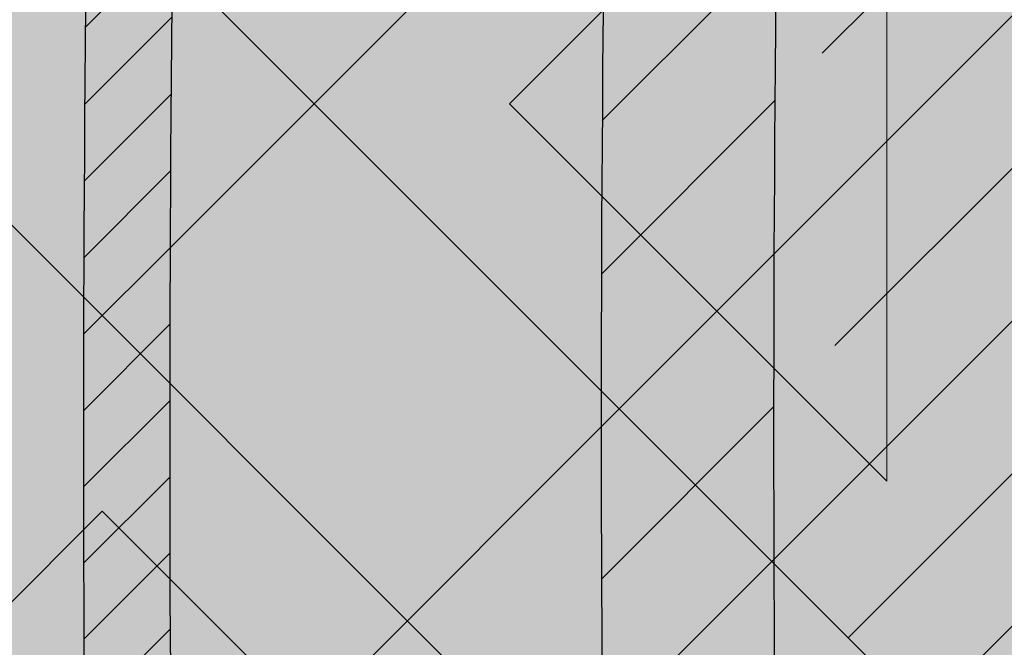
# Model space of a CAD drawing. Units: inches. Extents: x 844 to 2234, y 346 to 1084.
# Tile 11 of 93: x 1119.118 to 1120.937, y 693.702 to 694.861. Entities that reach past the tile are written whole.
import ezdxf

# ---------------------------------------------------------------- set-up
doc = ezdxf.new("R2010")
doc.units = ezdxf.units.IN
doc.header["$MEASUREMENT"] = 0
for name, color, linetype, lineweight in [('A-ANNO-DIMS', 2, 'Continuous', 18), ('furniture', 8, 'Continuous', 18), ('RA-AP-01$0$INT', 35, 'Continuous', 5)]:
    doc.layers.add(name, color=color, linetype=linetype, lineweight=lineweight)
doc.layers.add('RA-AP-01$0$FURN', color=3, linetype='Continuous')
doc.layers.add('RA-AP-01$0$WOOD', color=64, linetype='Continuous')
doc.styles.get("Standard").update_dxf_attribs({"font": 'arial.ttf'})
doc.dimstyles.get("Standard").update_dxf_attribs({"dimtxt": 6, "dimasz": 3, "dimexe": 0.18, "dimexo": 0.0625, "dimgap": 0.09, "dimtad": 0, "dimtih": 1, "dimtoh": 1, "dimdec": 1, "dimzin": 0, "dimdsep": 46, "dimlunit": 3, "dimtxsty": 'Standard', "dimblk": 'ARCHTICK', "dimcen": 0.09, "dimadec": 0, "dimazin": 0, "dimtfac": 1, "dimtdec": 1, "dimtofl": 0, "dimtmove": 0, "dimatfit": 3, "dimfxl": 1, "dimtolj": 1, "dimtzin": 0, "dimarcsym": 0})

# ---------------------------------------------------------------- blocks, each defined once
blk = doc.blocks.new('A$C18D01794')
at = {"layer": 'RA-AP-01$0$INT'}
h = blk.add_hatch(color=256, dxfattribs=at)
h.paths.add_polyline_path([(4.585917135068449, -6.356712009588271), (4.555206456959269, -6.35671200958746), (4.555206456959137, -6.387422687716308), (4.874495778835233, -6.706712009592356), (4.90520645695423, -6.676001331474049)])
h.paths.add_polyline_path([(5.255206456948813, -6.387422687716306), (5.255206456948682, -6.356712009605972), (5.224495778822613, -6.356712009605161), (4.905206456953498, -6.676001331474273), (4.935917135072151, -6.706712009592924)])
h.paths.add_polyline_path([(4.935917135072559, -6.706712009592068), (4.905206456953564, -6.737422687710376), (5.255206456951813, -7.087422687708613), (5.255206456951549, -7.026001331471008)])
h.paths.add_polyline_path([(4.555206456956399, -7.026001331471013), (4.555206456956134, -7.087422687708616), (4.905206456953821, -6.737422687710943), (4.874495778835166, -6.70671200959229)])
h = blk.add_hatch(color=256, dxfattribs=at)
h.paths.add_polyline_path([(4.585917135068448, -6.356712009588273), (4.614201406330596, -6.356712009589021), (4.668846067270487, -6.411356670531338), (4.723490728212344, -6.356712009591912), (4.771774999457151, -6.35671200959319), (4.826419660396886, -6.411356670535356), (4.862780050090322, -6.374996280843536), (4.844495778842715, -6.356712009595112), (4.862780050090411, -6.356712009595595), (4.905206456960182, -6.399138416468211), (4.947632863832445, -6.356712009597838), (4.965917135079675, -6.356712009598322), (4.947632863831759, -6.374996280845421), (4.983993253523576, -6.411356670538857), (5.038637914464627, -6.356712009600247), (5.08692218571208, -6.356712009601523), (5.141566846649976, -6.411356670541852), (5.196211507589851, -6.356712009604411), (5.224495778822615, -6.356712009605161), (4.905206456953975, -6.676001331473793)])
h.paths.add_polyline_path([(4.895206456956031, -6.637717060225675), (4.895206456958921, -6.528427738347902), (4.840561796018589, -6.583072399285802)], flags=16)
h.paths.add_polyline_path([(4.915206456955638, -6.637717060226121), (4.969851117895509, -6.583072399288678), (4.915206456957609, -6.528427738348344)], flags=16)
h.paths.add_polyline_path([(4.826419660395175, -6.568930263661755), (4.881064321335613, -6.514285602723745), (4.771774999456703, -6.514285602720857)], flags=16)
h.paths.add_polyline_path([(4.983993253519558, -6.568930263665262), (5.038637914460456, -6.514285602726792), (4.929348592581548, -6.514285602724816)], flags=16)
h.paths.add_polyline_path([(4.881064321336025, -6.494285602723742), (4.826419660397532, -6.439640941782821), (4.771774999457062, -6.494285602720859)], flags=16)
h.paths.add_polyline_path([(4.929348592582019, -6.494285602724817), (5.038637914460982, -6.494285602726792), (4.983993253522945, -6.439640941786327)], flags=16)
h.paths.add_polyline_path([(4.895206456960191, -6.480143467100443), (4.895206456962115, -6.407422687715913), (4.876922185715016, -6.389138416467584), (4.840561796021581, -6.425498806159401)], flags=16)
h.paths.add_polyline_path([(4.915206456958487, -6.480143467100889), (4.969851117899527, -6.425498806162279), (4.933490728206909, -6.389138416468043), (4.9152064569598, -6.40742268771434)], flags=16)
h.paths.add_polyline_path([(4.757632863832376, -6.480143467096812), (4.812277524772842, -6.425498806158772), (4.757632863834348, -6.370854145217844)], flags=16)
h.paths.add_polyline_path([(4.737632863832376, -6.480143467096286), (4.737632863834348, -6.370854145217375), (4.682988202893906, -6.425498806155385)], flags=16)
h.paths.add_polyline_path([(5.05278005008503, -6.480143467103376), (5.052780050087917, -6.370854145224413), (4.998135389146995, -6.425498806162908)], flags=16)
h.paths.add_polyline_path([(5.072780050085024, -6.480143467103744), (5.127424711025931, -6.42549880616527), (5.072780050087916, -6.370854145224832)], flags=16)
h.paths.add_polyline_path([(4.935917135072783, -6.706712009592292), (5.255206456948811, -6.387422687716309), (5.255206456948932, -6.415706958964177), (5.200561796010279, -6.470351619902839), (5.255206456949403, -6.524996280841948), (5.25520645694961, -6.5732805520894), (5.200561796009787, -6.627925213029239), (5.236922185702417, -6.664285602721864), (5.255206456949919, -6.646001331474357), (5.255206456949998, -6.664285602721898), (5.212780050078687, -6.706712009592262), (5.25520645695036, -6.749138416463932), (5.255206456950438, -6.767422687711313), (5.236922185702424, -6.749138416463297), (5.200561796009796, -6.785498806155928), (5.255206456950753, -6.840143467096874), (5.25520645695096, -6.888427738341682), (5.200561796010322, -6.943072399282328), (5.255206456951428, -6.997717060223427), (5.255206456951547, -7.026001331471006)])
h.paths.add_polyline_path([(5.042988202883395, -6.785498806155427), (5.097632863823085, -6.840143467095101), (5.097632863822622, -6.730854145216193)], flags=16)
h.paths.add_polyline_path([(5.028846067259663, -6.771356670531693), (5.083490728198774, -6.716712009592573), (4.974201406321001, -6.716712009593042)], flags=16)
h.paths.add_polyline_path([(5.117632863823087, -6.840143467095186), (5.172277524762331, -6.785498806155926), (5.11763286382262, -6.730854145216225)], flags=16)
h.paths.add_polyline_path([(5.08349072819877, -6.696712009593886), (5.028846067259652, -6.642067348654775), (4.974201406320998, -6.696712009593438)], flags=16)
h.paths.add_polyline_path([(5.131774999446817, -6.854285602718917), (5.186419660386065, -6.799640941779662), (5.241064321325782, -6.854285602719365)], flags=17)
h.paths.add_polyline_path([(5.131774999446228, -6.716712009592374), (5.186419660386065, -6.771356670532194), (5.222780050079488, -6.734996280838764), (5.204495778832781, -6.716712009592063)], flags=16)
h.paths.add_polyline_path([(5.097632863822613, -6.682569873970264), (5.097632863823061, -6.573280552091354), (5.042988202883383, -6.627925213031044)], flags=16)
h.paths.add_polyline_path([(5.131774999446899, -6.874285602718915), (5.241064321325809, -6.874285602719364), (5.186419660386591, -6.928930263658598)], flags=17)
h.paths.add_polyline_path([(5.131774999446226, -6.696712009594078), (5.204495778830767, -6.696712009594374), (5.22278005007868, -6.67842773834687), (5.186419660386049, -6.642067348654249)], flags=16)
h.paths.add_polyline_path([(5.11763286382262, -6.682569873970225), (5.17227752476232, -6.627925213030515), (5.117632863823064, -6.573280552091267)], flags=16)
h.paths.add_polyline_path([(5.186419660386069, -6.613783077405491), (5.241064321325754, -6.559138416465795), (5.131774999446791, -6.559138416466263)], flags=16)
h.paths.add_polyline_path([(5.131774999446872, -6.539138416466263), (5.24106432132578, -6.539138416465794), (5.186419660386554, -6.484493755526573)], flags=16)
h.paths.add_polyline_path([(5.255206456951811, -7.08742268770861), (5.255206456951895, -7.106712009588038), (4.555206456956052, -7.106712009588038), (4.555206456956136, -7.087422687708617), (4.905206456953973, -6.737422687710788)])
h.paths.add_polyline_path([(4.983993253513404, -6.8444937555241), (4.92934859257295, -6.899138416462108), (5.03863791445186, -6.899138416465014)], flags=16)
h.paths.add_polyline_path([(4.969851117889988, -6.83035161990006), (4.915206456952556, -6.775706958960171), (4.915206456949648, -6.884996280837944)], flags=16)
h.paths.add_polyline_path([(4.929348592572535, -6.919138416462105), (4.983993253511019, -6.973783077403037), (5.038637914451496, -6.919138416465012)], flags=16)
h.paths.add_polyline_path([(5.052780050074912, -6.93328055208906), (4.998135389134438, -6.987925213027088), (5.052780050072919, -7.042569873968025)], flags=16)
h.paths.add_polyline_path([(5.07278005007491, -6.933280552089588), (5.072780050072918, -7.042569873968497), (5.127424711013374, -6.987925213030498)], flags=16)
h.paths.add_polyline_path([(4.89520645695295, -6.775706958959721), (4.840561796013067, -6.830351619897157), (4.895206456950961, -6.884996280837494)], flags=16)
h.paths.add_polyline_path([(4.915206456948365, -6.933280552085403), (4.915206456946434, -7.006001331471951), (4.933490728192729, -7.024285602719066), (4.969851117886972, -6.987925213026453)], flags=16)
h.paths.add_polyline_path([(4.881064321327021, -6.899138416461022), (4.82641966038902, -6.84449375552057), (4.771774999448108, -6.899138416459029)], flags=16)
h.paths.add_polyline_path([(4.895206456950073, -6.933280552084951), (4.840561796009022, -6.987925213023558), (4.876922185700835, -7.024285602716997), (4.895206456948749, -7.006001331469487)], flags=16)
h.paths.add_polyline_path([(4.983993253510392, -7.0020673486505), (4.947632863816944, -7.038427738342319), (4.965917135064043, -7.05671200959023), (5.038637914448995, -7.056712009591555)], flags=16)
h.paths.add_polyline_path([(4.881064321326543, -6.91913841646102), (4.771774999447578, -6.919138416459031), (4.826419660385607, -6.973783077399508)], flags=16)
h.paths.add_polyline_path([(4.905206456946447, -7.014285602717636), (4.862780050074785, -7.056712009588352), (4.947632863816685, -7.056712009589775)], flags=16)
h.paths.add_polyline_path([(5.14156684663679, -7.002067348654549), (5.086922185696452, -7.056712009592438), (5.196211507574223, -7.056712009594425)], flags=16)
h.paths.add_polyline_path([(4.8264196603837, -7.002067348646972), (4.771774999442643, -7.056712009585575), (4.8444957788276, -7.056712009587508), (4.862780050075511, -7.038427738340416)], flags=16)
h.paths.add_polyline_path([(4.812277524760289, -6.98792521302292), (4.757632863822258, -6.933280552082447), (4.757632863819352, -7.042569873961408)], flags=16)
h.paths.add_polyline_path([(4.73763286382226, -6.933280552082079), (4.682988202881349, -6.987925213020536), (4.737632863819352, -7.04256987396099)], flags=16)
h.paths.add_polyline_path([(4.723490728195188, -7.056712009584289), (4.668846067257299, -7.002067348643949), (4.614201406317417, -7.056712009581383)], flags=16)
h.paths.add_polyline_path([(4.597632863829262, -6.706712009592262), (4.555206456957951, -6.664285602721896), (4.555206456958029, -6.646001331474357), (4.573490728205535, -6.664285602721864), (4.609851117898167, -6.627925213029238), (4.555206456958338, -6.573280552089402), (4.555206456958546, -6.524996280841952), (4.60985111789767, -6.470351619902839), (4.555206456959015, -6.415706958964177), (4.555206456959138, -6.387422687716309), (4.874495778835167, -6.70671200959229), (4.5552064569564, -7.026001331471015), (4.555206456956523, -6.997717060223433), (4.609851117897629, -6.94307239928233), (4.555206456956988, -6.888427738341681), (4.555206456957198, -6.840143467096881), (4.609851117898153, -6.78549880615593), (4.573490728205528, -6.749138416463297), (4.555206456957507, -6.76742268771132), (4.555206456957585, -6.749138416463933)])
h.paths.add_polyline_path([(4.712780050085332, -6.730854145216195), (4.712780050084863, -6.840143467095105), (4.767424711024555, -6.785498806155427)], flags=16)
h.paths.add_polyline_path([(4.726922185709173, -6.716712009592573), (4.781566846648288, -6.771356670531693), (4.836211507586949, -6.716712009593043)], flags=16)
h.paths.add_polyline_path([(4.692780050085327, -6.730854145216225), (4.638135389145619, -6.785498806155928), (4.692780050084865, -6.840143467095185)], flags=16)
h.paths.add_polyline_path([(4.726922185709182, -6.696712009593886), (4.836211507586949, -6.696712009593436), (4.7815668466483, -6.642067348654773)], flags=16)
h.paths.add_polyline_path([(4.678637914461726, -6.71671200959237), (4.605917135075169, -6.716712009592063), (4.587632863828464, -6.734996280838766), (4.623993253521887, -6.771356670532195)], flags=16)
h.paths.add_polyline_path([(4.712780050085336, -6.68256987397026), (4.767424711024568, -6.627925213031042), (4.71278005008489, -6.573280552091352)], flags=16)
h.paths.add_polyline_path([(4.678637914461726, -6.696712009594076), (4.623993253521899, -6.642067348654247), (4.587632863829271, -6.67842773834687), (4.605917135077185, -6.696712009594376)], flags=16)
h.paths.add_polyline_path([(4.692780050085336, -6.682569873970228), (4.692780050084889, -6.573280552091267), (4.638135389145632, -6.627925213030515)], flags=16)
h.paths.add_polyline_path([(4.623993253521885, -6.799640941779662), (4.678637914461131, -6.854285602718915), (4.56934859258217, -6.854285602719365)], flags=17)
h.paths.add_polyline_path([(4.623993253521901, -6.613783077405509), (4.678637914461158, -6.559138416466263), (4.569348592582195, -6.559138416465795)], flags=16)
h.paths.add_polyline_path([(4.678637914461051, -6.874285602718915), (4.623993253521361, -6.928930263658598), (4.569348592582143, -6.874285602719364)], flags=17)
h.paths.add_polyline_path([(4.678637914461076, -6.539138416466263), (4.623993253521399, -6.484493755526573), (4.569348592582167, -6.539138416465796)], flags=16)
h = blk.add_hatch(color=256, dxfattribs=at)
h.paths.add_polyline_path([(4.781566846647504, -6.771356670530272), (4.836211507586161, -6.716712009591613), (4.726922185708388, -6.716712009591159)])
h.paths.add_polyline_path([(4.836211507586161, -6.696712009592008), (4.781566846647504, -6.642067348653354), (4.726922185708388, -6.69671200959247)])
h.paths.add_polyline_path([(4.76742471102377, -6.627925213029623), (4.712780050084083, -6.57328055208994), (4.712780050084542, -6.68256987396885)])
h.paths.add_polyline_path([(4.692780050084544, -6.682569873968819), (4.692780050084084, -6.573280552089856), (4.638135389144834, -6.627925213029111)])
h.paths.add_polyline_path([(4.678637914460932, -6.696712009592669), (4.623993253521102, -6.642067348652844), (4.587632863827676, -6.678427738346266), (4.605917135074382, -6.696712009592973)])
h.paths.add_polyline_path([(4.573490728204743, -6.664285602721736), (4.60985111789737, -6.627925213029108), (4.555206456957541, -6.573280552089279), (4.555206456957237, -6.646001331474231)])
h.paths.add_polyline_path([(4.623993253521098, -6.613783077405377), (4.67863791446035, -6.559138416466126), (4.56934859258139, -6.559138416465669)])
h.paths.add_polyline_path([(4.678637914460275, -6.539138416466126), (4.623993253520583, -6.48449375552644), (4.56934859258136, -6.539138416465672)])
h.paths.add_polyline_path([(4.609851117896854, -6.470351619902707), (4.555206456958196, -6.415706958964051), (4.555206456957738, -6.524996280841822)])
h.paths.add_polyline_path([(4.597632863828475, -6.706712009592775), (4.555206456957283, -6.664285602721582), (4.555206456956805, -6.749138416463489)])
h.paths.add_polyline_path([(4.678637914460932, -6.716712009590963), (4.605917135076396, -6.71671200959066), (4.587632863828479, -6.734996280838164), (4.623993253521104, -6.771356670530792)])
h.paths.add_polyline_path([(4.692780050084091, -6.840143467093776), (4.692780050084548, -6.730854145214809), (4.638135389144834, -6.785498806154524)])
h.paths.add_polyline_path([(4.767424711023772, -6.785498806154004), (4.712780050084545, -6.730854145214786), (4.712780050084089, -6.840143467093692)])
h.paths.add_polyline_path([(4.67863791446036, -6.854285602718778), (4.623993253521105, -6.799640941779527), (4.569348592581399, -6.854285602719237)])
h.paths.add_polyline_path([(4.609851117897371, -6.785498806155798), (4.573490728204743, -6.74913841646317), (4.555206456957237, -6.767422687710675), (4.555206456957548, -6.840143467095629)])
h.paths.add_polyline_path([(4.623993253520596, -6.928930263658465), (4.67863791446028, -6.874285602718778), (4.569348592581367, -6.874285602719238)])
h.paths.add_polyline_path([(4.609851117896867, -6.943072399282199), (4.555206456957749, -6.888427738343082), (4.55520645695821, -6.997717060220857)])
h = blk.add_hatch(color=256, dxfattribs=at)
h.paths.add_polyline_path([(4.895206456952951, -6.77570695895972), (4.840561796013068, -6.830351619897156), (4.895206456950958, -6.884996280837495)])
h.paths.add_polyline_path([(4.915206456949649, -6.884996280837942), (4.969851117889987, -6.830351619900054), (4.915206456952556, -6.775706958960171)])
h.paths.add_polyline_path([(5.038637914451862, -6.899138416465013), (4.983993253513403, -6.8444937555241), (4.929348592572953, -6.899138416462106)])
h.paths.add_polyline_path([(4.929348592572535, -6.919138416462105), (4.983993253511018, -6.973783077403037), (5.038637914451497, -6.919138416465012)])
h.paths.add_polyline_path([(4.915206456948366, -6.933280552085397), (4.915206456946433, -7.006001331471951), (4.93349072819273, -7.024285602719068), (4.969851117886972, -6.987925213026454)])
h.paths.add_polyline_path([(5.038637914448995, -7.056712009591553), (4.983993253510389, -7.002067348650502), (4.947632863816946, -7.038427738342318), (4.965917135064043, -7.05671200959023)])
h.paths.add_polyline_path([(5.05278005007292, -7.042569873968023), (5.05278005007491, -6.933280552089059), (4.998135389134438, -6.987925213027088)])
h.paths.add_polyline_path([(5.07278005007292, -7.042569873968496), (5.127424711013374, -6.987925213030498), (5.072780050074909, -6.933280552089588)])
h.paths.add_polyline_path([(5.141566846636789, -7.002067348654547), (5.086922185696449, -7.056712009592438), (5.196211507574223, -7.056712009594425)])
h.paths.add_polyline_path([(4.947632863816688, -7.056712009589774), (4.905206456946449, -7.014285602717634), (4.862780050074784, -7.056712009588353)])
h.paths.add_polyline_path([(4.840561796009025, -6.987925213023556), (4.876922185700834, -7.024285602716997), (4.895206456948747, -7.006001331469488), (4.895206456950075, -6.933280552084953)])
h.paths.add_polyline_path([(4.88106432132654, -6.919138416461021), (4.771774999447577, -6.919138416459031), (4.826419660385606, -6.973783077399508)])
h.paths.add_polyline_path([(4.881064321327019, -6.899138416461022), (4.826419660389019, -6.844493755520571), (4.771774999448108, -6.89913841645903)])
h.paths.add_polyline_path([(4.757632863819352, -7.042569873961409), (4.812277524760284, -6.987925213022922), (4.757632863822259, -6.933280552082447)])
h.paths.add_polyline_path([(4.8264196603837, -7.002067348646974), (4.771774999442646, -7.056712009585575), (4.844495778827599, -7.05671200958751), (4.862780050075512, -7.038427738340417)])
h.paths.add_polyline_path([(4.737632863819352, -7.042569873960988), (4.737632863822258, -6.933280552082078), (4.682988202881349, -6.987925213020538)])
h.paths.add_polyline_path([(4.668846067257299, -7.002067348643952), (4.61420140631742, -7.056712009581384), (4.723490728195189, -7.056712009584292)])
for p, q in [((4.874495778835167, -6.70671200959229), (4.555206456956399, -7.026001331471013)), ((4.905206456953975, -6.737422687710788), (4.555206456956136, -7.087422687708617)), ((4.569348592582142, -6.874285602719364), (4.623993253521361, -6.928930263658598)), ((4.623993253521363, -6.928930263658596), (4.678637914461051, -6.874285602718915)), ((4.682988202881351, -6.987925213020536), (4.737632863822258, -6.933280552082079)), ((4.737632863822258, -6.933280552082079), (4.737632863819352, -7.042569873960989)), ((4.737632863819352, -7.042569873960989), (4.682988202881349, -6.987925213020538))]:
    blk.add_line(p, q, dxfattribs=at)
blk = doc.blocks.new('A$C32926AE1')
at = {"layer": 'RA-AP-01$0$FURN'}
h = blk.add_hatch(dxfattribs=at)
h.set_pattern_fill('ANSI31', color=256, scale=0.1, style=0)
h.set_pattern_definition([(45, (0, 0), (-0.0088388347648318, 0.0088388347648318), [])])
edge = h.paths.add_edge_path(flags=16)
edge.add_arc((4.904771284329206, 4.246793130718756), 0.2603971832811541, 75.22398030683196, 104.7760196931204)
edge.add_arc((4.904771284329206, 4.246793130718756), 0.2603971832811541, 75.223980306832, 104.77601969312039, ccw=False)
edge = h.paths.add_edge_path(flags=16)
edge.add_arc((4.904771284329206, 4.067062675376612), 0.2603971832811541, 255.2239803068796, 284.776019693168)
edge.add_arc((4.904771284329206, 4.067062675376612), 0.2603971832811541, 255.22398030687958, 284.77601969316805, ccw=False)
edge = h.paths.add_edge_path(flags=0)
edge.add_arc((4.904771284329206, 4.067062675376612), 0.2603971832811541, 255.2239803068796, 284.776019693168)
edge.add_arc((4.904771284329206, 4.067062675376612), 0.2603971832811541, 255.22398030687958, 284.77601969316805, ccw=False)
edge = h.paths.add_edge_path(flags=0)
edge.add_arc((4.904771284329206, 4.067062675376612), 0.2603971832811541, 255.2239803068796, 284.776019693168)
edge.add_arc((4.904771284329206, 4.067062675376612), 0.2603971832811541, 255.22398030687958, 284.77601969316805, ccw=False)
edge = h.paths.add_edge_path()
edge.add_arc((4.604388392048174, 4.588829985554312), 0.1599999999999918, 342.3781640246255, 354.4317409793762)
edge.add_arc((5.090145208887507, 4.43216705527679), 0.3503971832811637, 162.0091218307731, 180.3186872093483)
edge.add_arc((5.205154176610243, 4.588829985554953), 0.1599999999999917, 185.5682590208461, 197.6218359767349)
edge.add_arc((4.904771284329229, 4.246793130718735), 0.3503971832811761, 72.00912183053516, 107.9908781690354)
edge.add_arc((9.535952835716557, 4.28682295566602), 4.798342501046485, 178.2875002453811, 181.5576802719453)
edge.add_arc((4.719397359771122, 4.43216705527679), 0.3503971832811637, 359.6813127906516, 377.9908781692269)
edge.add_arc((9.535967292294904, 4.286822350292874), 4.778371420254705, 178.2965938931842, 181.5667745797229)
edge.add_arc((4.719397359771122, 4.43216705527679), 0.3303971832811637, 359.6813127906516, 377.9908781692269)
edge.add_arc((0.2735752763637294, 4.286822350292874), 4.7783714202547, 358.4332254202771, 361.7034061068158)
edge.add_arc((5.061434214606998, 4.732549947558029), 0.1600000000000254, 252.3781640250584, 264.4317409792362)
edge.add_arc((4.748108354051257, 4.732549947558012), 0.1600000000000541, 275.5682590208426, 287.6218359759532)
edge.add_arc((4.604388392048115, 4.588829985554317), 0.1800000000000505, 342.3567572500182, 349.3735009646207)
edge.add_arc((5.205154176610254, 4.588829985554976), 0.1800000000000069, 190.6264990356027, 197.6432427513933)
edge.add_arc((5.061434214607106, 4.732549947558013), 0.1800000000000424, 252.3567572496606, 259.3735009644582)
edge.add_arc((4.904771284329208, 4.246793130718737), 0.3303971832811676, 71.99844483668534, 108.0015551637021)
edge.add_arc((4.748108354051414, 4.732549947558045), 0.1800000000000547, 280.6264990355479, 287.6432427495938)
edge.add_arc((5.090145208887514, 4.432167055276789), 0.2803971832811691, 162.8706300666893, 180.816523289902)
edge.add_arc((4.719397359771136, 4.432167055276689), 0.2803971832811534, 359.183476710103, 377.1293699333214)
edge.add_arc((4.904771284329222, 4.246793130718737), 0.2803971832811769, 72.87063006672916, 107.1293699332334)
edge.add_arc((5.090145208887522, 4.432167055276788), 0.2603971832811776, 165.2239803068007, 180.9953123810312)
edge.add_arc((4.719397359771141, 4.432167055276699), 0.2603971832811458, 359.0046876189768, 374.7760196932087)
edge.add_arc((5.090145208887507, 4.43216705527679), 0.3303971832811637, 162.0091218307731, 180.3186872093483)
edge.add_arc((9.53595427642584, 4.285015535491528), 4.728345371032053, 178.265043920078, 181.5679956281801)
edge.add_arc((0.2735882922327999, 4.285015535491582), 4.728345371032045, 358.4320043718193, 361.7349560799204)
edge.add_arc((9.535953591267507, 4.284458026472751), 4.708343996644348, 178.2573054306777, 181.5704995759608)
edge.add_arc((0.273588977391114, 4.284458026472785), 4.708343996644358, 358.4295004240388, 361.7426945693213)
edge.add_arc((0.2735889773911131, 4.029397779622582), 4.708343996644359, 358.2573054306787, 361.5704995759613)
edge.add_arc((9.535953591267518, 4.029397779622618), 4.708343996644359, 178.4295004240391, 181.7426945693223)
edge.add_arc((0.2735882922327901, 4.028840270603786), 4.728345371032054, 358.2650439200796, 361.5679956281808)
edge.add_arc((9.53595427642584, 4.028840270603841), 4.728345371032054, 178.4320043718199, 181.7349560799219)
edge.add_arc((0.2735752763637302, 4.027033455802493), 4.778371420254699, 358.2965938931842, 361.5667745797229)
edge.add_arc((4.719397359771122, 3.881688750818578), 0.3303971832811637, 342.0091218307731, 360.3186872093484)
edge.add_arc((5.090145208887507, 3.881688750818578), 0.3303971832811637, 179.6813127906516, 197.9908781692269)
edge.add_arc((9.535967292294904, 4.027033455802493), 4.778371420254705, 178.433225420277, 181.7034061068158)
edge.add_arc((4.719397359771122, 3.881688750818578), 0.3503971832811637, 342.0091218307731, 360.3186872093484)
edge.add_arc((9.53595283571655, 4.027032850429349), 4.79834250104648, 178.4423197280546, 181.7124997546188)
edge.add_arc((4.719397359771141, 3.881688750818669), 0.2603971832811458, 345.2239803067913, 360.9953123810232)
edge.add_arc((5.090145208887522, 3.88168875081858), 0.2603971832811776, 179.0046876189687, 194.7760196931993)
edge.add_arc((4.904771284329222, 4.067062675376631), 0.2803971832811769, 252.8706300667665, 287.1293699332708)
edge.add_arc((4.719397359771136, 3.881688750818678), 0.2803971832811534, 342.8706300666787, 360.8165232898969)
edge.add_arc((5.090145208887514, 3.881688750818579), 0.2803971832811691, 179.183476710098, 197.1293699333106)
edge.add_arc((4.748108354051414, 3.581305858537323), 0.1800000000000547, 72.3567572504062, 79.37350096445199)
edge.add_arc((4.904771284329208, 4.067062675376631), 0.3303971832811676, 251.9984448362979, 288.0015551633146)
edge.add_arc((5.061434214607106, 3.581305858537355), 0.1800000000000424, 100.6264990355418, 107.6432427503394)
edge.add_arc((5.205154176610254, 3.725025820540392), 0.1800000000000069, 162.3567572486066, 169.3735009643972)
edge.add_arc((4.604388392048115, 3.725025820541051), 0.1800000000000505, 10.62649903537925, 17.64324274998182)
edge.add_arc((4.748108354051257, 3.581305858537356), 0.1600000000000541, 72.37816402404681, 84.43174097915735)
edge.add_arc((4.904771284329229, 4.067062675376632), 0.3503971832811761, 252.0091218309645, 287.9908781694648)
edge.add_arc((5.061434214606998, 3.581305858537339), 0.1600000000000254, 95.56825902076373, 107.6218359749416)
edge.add_arc((5.205154176610243, 3.725025820540414), 0.1599999999999917, 162.3781640232651, 174.4317409791539)
edge.add_arc((5.090145208887507, 3.881688750818578), 0.3503971832811637, 179.6813127906516, 197.9908781692269)
edge.add_arc((4.604388392048174, 3.725025820541056), 0.1599999999999918, 5.568259020623824, 17.62183597537444)
edge.add_arc((0.2735897329420762, 4.28682295566602), 4.798342501046482, 358.4423197280547, 361.7124997546188)
edge.add_arc((0.2735897329420691, 4.027032850429348), 4.798342501046489, 358.2875002453812, 361.5576802719453)
at = {"layer": 'RA-AP-01$0$WOOD'}
h = blk.add_hatch(color=256, dxfattribs=at)
h.dxf.hatch_style = 1
h.paths.add_polyline_path([(5.157430609644524, 4.573483066760929, -0.1009492694046607), (5.155401577623758, 4.593365984175333, -0.1842662638101597), (5.172249623284174, 4.638795604568598, 0.2056608120311276), (5.179560981299304, 4.661316324430096, 0.3614336704623542), (5.134352340494423, 4.706524965234944, 0.2056608120311297), (5.111831620632933, 4.699213607219793, -0.1842662638101113), (5.066402000239693, 4.682365561559342, -0.1055311479399994), (5.045656153913092, 4.68467289944697, 0.1567636581983829), (4.763886414745334, 4.684672899446966, -0.1055311479399895), (4.743140568418733, 4.68236556155934, -0.1842662638100833), (4.6977109480255, 4.69921360721979, 0.2056608120302612), (4.675190228164109, 4.706524965234949, 0.3614336704708441), (4.629981587358889, 4.66131632442871, 0.2056608120245944), (4.637292945374126, 4.638795604567974, -0.1842662638101024), (4.654140991034615, 4.59336598417475, -0.1009492694055169), (4.652111959013835, 4.573483066760181, 0.021410119221476), (4.629748025606143, 4.156712009541676, 0.0214101192214795), (4.652111959013809, 3.739940952323101, -0.1009492694059586), (4.654140991034615, 3.720058034908448, -0.1842662638100975), (4.637292945374126, 3.674628414515226, 0.2056608120245705), (4.629981587358889, 3.652107694654492, 0.3614336704708879), (4.675190228164113, 3.606899053848249, 0.2056608120302384), (4.697710948025501, 3.614210411863408, -0.1842662638100995), (4.743140568418738, 3.63105845752386, -0.1055311479402541), (4.763886414745388, 3.628751119636215, 0.1567636581983776), (5.045656153913137, 3.628751119636244, -0.1055311479397538), (5.066402000239692, 3.631058457523857, -0.1842662638101067), (5.111831620632931, 3.614210411863407, 0.2056608120310924), (5.134352340494417, 3.606899053848256, 0.3614336704624001), (5.179560981299307, 3.652107694653103, 0.2056608120311314), (5.172249623284175, 3.6746284145146, -0.1842662638101402), (5.155401577623758, 3.72005803490786, -0.1009492694051366), (5.15743060964455, 3.739940952322354, 0.0214101192215073), (5.179794543052287, 4.156712009541468, 0.0214101192215252)])
h.paths.add_polyline_path([(4.639748609479751, 4.156712009541513, 0.0213537860821624), (4.661970494867118, 3.741887061152232, -0.094075836301374), (4.664143710413708, 3.7196126951003, -0.1824818158568985), (4.644813765429836, 3.668037719127816, 0.2056608120245319), (4.639939526753007, 3.653023905887301, 0.3614336704710246), (4.676106439397173, 3.616856993242342, 0.2056608120302234), (4.691120252638095, 3.621731231919122, -0.1824818158602558), (4.742695228611606, 3.641061176902986, -0.1029891339458722), (4.766991894714349, 3.638256818950944, 0.156709409989566), (5.042550673941472, 3.638256818950105, -0.102989133958497), (5.066847340047078, 3.641061176902949, -0.1824818158594995), (5.118422316020358, 3.621731231919103, 0.2056608120311416), (5.133436129261316, 3.616856993242346, 0.3614336704621468), (5.169603041905217, 3.653023905886178, 0.2056608120310986), (5.164728803228477, 3.668037719127177, -0.1824818158565612), (5.145398858244737, 3.719612695099578, -0.0940758363009313), (5.147572073791232, 3.741887061151398, 0.0213537860822023), (5.169793959178681, 4.156712009541451, 0.0213537860822226), (5.147572073791203, 4.571536957931898, -0.0940758363005034), (5.145398858244737, 4.59381132398362, -0.1824818158565587), (5.164728803228476, 4.645386299956021, 0.2056608120311045), (5.169603041905216, 4.66040011319702, 0.3614336704621845), (5.133436129261313, 4.696567025840856, 0.2056608120310773), (5.118422316020359, 4.691692787164098, -0.182481815859508), (5.066847340047078, 4.67236284218025, -0.1029891339584606), (5.04255067394148, 4.675167200133092, 0.156709409989566), (4.766991894714357, 4.675167200132257, -0.1029891339458842), (4.742695228611611, 4.672362842180213, -0.1824818158602725), (4.691120252638095, 4.691692787164077, 0.2056608120302152), (4.676106439397174, 4.696567025840858, 0.3614336704710363), (4.639939526753005, 4.660400113195899, 0.2056608120245495), (4.644813765429837, 4.645386299955384, -0.1824818158568934), (4.664143710413708, 4.593811323982902, -0.0940758363009187), (4.661970494867149, 4.571536957931074, 0.021353786082177)], flags=16)
h.paths.add_polyline_path([(5.129794543052235, 4.432167055276933, -0.0141661062790638), (5.130152669293814, 4.156927903047693, -0.0141661062790647), (5.129794543052234, 3.881688750818433, -0.0785247771143638), (5.10979738006795, 3.755143611847103, 0.0945969212073497), (5.105408519571111, 3.717898134952927, 0.1043170707844957), (5.116074640131521, 3.670385395016088, 0.1043170707864965), (5.068561900193738, 3.681051515576561, 0.09459692119553), (5.031316423304057, 3.676662655080835, -0.1580239521427272), (4.778226145355827, 3.676662655080367, 0.0945969211986668), (4.740980668464973, 3.681051515576592, 0.1043170707882822), (4.693467928526415, 3.670385395015844, 0.1043170707867916), (4.704134049087309, 3.717898134953662, 0.0945969211972894), (4.69974518859162, 3.755143611844042, -0.0785247771163196), (4.679748025606343, 3.881688750818406, -0.0141661062790663), (4.679389899364763, 4.156927903047693, -0.0141661062790672), (4.679748025606343, 4.432167055276998, -0.0785247771163064), (4.699745188591625, 4.55871219425134, 0.094596921197333), (4.704134049087308, 4.595957671141738, 0.1043170707867205), (4.693467928526416, 4.643470411079523, 0.1043170707882628), (4.740980668464965, 4.632804290518776, 0.0945969211988114), (4.778226145355874, 4.637193151015016, -0.158023952142669), (5.031316423304015, 4.637193151014546, 0.0945969211956361), (5.068561900193736, 4.632804290518806, 0.1043170707864979), (5.11607464013152, 4.643470411079278, 0.1043170707844617), (5.105408519571112, 4.595957671142455, 0.0945969212074597), (5.109797380067959, 4.558712194248236, -0.0785247771143467)], flags=0)
h.paths.add_polyline_path([(5.119794532311105, 4.432259799204851, -0.0142000800617244), (5.120156169157484, 4.156927903047701, -0.0142000800617277), (5.119794532311105, 3.881596006890482, -0.0784894509520253), (5.100273383573699, 3.758192358677797, 0.0940138827242913), (5.095413455884425, 3.717477693979438, 0.0606271852308753), (5.099615656341024, 3.686844378806616, 0.0606271852322524), (5.068982341167493, 3.691046579263239, 0.0940138827010453), (5.028267676478798, 3.686186651576848, -0.1580706864508061), (4.781274892180912, 3.686186651576435, 0.0940138827026903), (4.740560227491556, 3.691046579263279, 0.0606271852339895), (4.709926912317155, 3.686844378806508, 0.0606271852329405), (4.714129112773991, 3.717477693980356, 0.094013882701304), (4.709269185087677, 3.758192358669163, -0.0784894509577193), (4.689748036347473, 3.881596006890469, -0.014200080061729), (4.689386399501094, 4.156927903047709, -0.0142000800617217), (4.689748036347473, 4.432259799204808, -0.078489450957724), (4.709269185087651, 4.555663447426125, 0.0940138827014585), (4.714129112773992, 4.596378112114996, 0.0606271852329731), (4.709926912317154, 4.62701142728886, 0.0606271852340196), (4.74056022749157, 4.622809226832087, 0.0940138827024997), (4.781274892180847, 4.627669154518912, -0.1580706864508359), (5.028267676478777, 4.627669154518526, 0.0940138827010946), (5.068982341167492, 4.622809226832129, 0.060627185232254), (5.099615656341024, 4.627011427288751, 0.0606271852308727), (5.095413455884425, 4.59637811211593, 0.0940138827241088), (5.100273383573675, 4.555663447417647, -0.0784894509520978)], flags=0)
h.paths.add_polyline_path([(5.06978912287499, 4.430218106756144, -0.014241683694547), (5.070173729147532, 4.156927903047672, -0.0142416836945458), (5.06978912287499, 3.883637699339223, -0.0800609523125196), (5.052662118612511, 3.773463122773442, 0.0526421978001116), (5.04590916754064, 3.740550867606997, 0.0526421977992423), (5.012996912374707, 3.73379791653534, -0.1583028414718258), (4.796545656286308, 3.73379791653451, 0.0526421978034211), (4.763633401117837, 3.740550867607021, 0.0526421978018622), (4.756880450045755, 3.773463122774558, -0.0800609523117106), (4.739753445783639, 3.883637699339268, -0.0142416836945435), (4.739368839511098, 4.156927903047671, -0.0142416836945477), (4.739753445783639, 4.430218106756155, -0.0800609523116345), (4.75688045004574, 4.540392683320762, 0.052642197801941), (4.763633401117837, 4.573304938488346, 0.0526421978035071), (4.796545656286361, 4.580057889560873, -0.1583028414717561), (5.012996912374669, 4.580057889560039, 0.0526421977993048), (5.04590916754064, 4.57330493848837, 0.0526421978002057), (5.052662118612529, 4.540392683321868, -0.080060952312477)], flags=0)
h.paths.add_polyline_path([(5.049789715110557, 4.43038092723357, -0.0143097550741839), (5.05018085590259, 4.156927903047715, -0.0143097550741854), (5.049789715110558, 3.883474878861827, -0.0800685599149176), (5.03362098255317, 3.779581877367999, 0.0306258898956367), (5.028241146483733, 3.758218888663947, 0.0306258898977031), (5.006878157778253, 3.75283905259408, -0.1583983521624096), (4.802664410878162, 3.752839052594731, 0.0306258898946014), (4.781301422174808, 3.758218888663924, 0.0306258898967912), (4.775921586105202, 3.779581877368794, -0.080068559914251), (4.759752853548071, 3.883474878861786, -0.0143097550741854), (4.759361712756037, 4.156927903047671, -0.0143097550741854), (4.759752853548071, 4.430380927233557, -0.0800685599142479), (4.775921586105193, 4.534273928726546, 0.0306258898968306), (4.781301422174808, 4.555636917431444, 0.0306258898945754), (4.802664410878143, 4.561016753500631, -0.1583983521624168), (5.006878157778244, 4.561016753501291, 0.0306258898977177), (5.028241146483733, 4.555636917431421, 0.0306258898958182), (5.03362098255321, 4.534273928727244, -0.080068559914796)], flags=0)
h.paths.add_polyline_path([(4.999766070382627, 4.428171244713864, -0.0143443147609634), (5.000198441819402, 4.156927903047689, -0.0143443147609612), (4.999766070382627, 3.885684561381556, -0.0784641635803329), (4.987356730658798, 3.799103304488872, -0.1506053783831347), (4.822185837999821, 3.79910330448882, -0.0784641635803318), (4.809776498276007, 3.885684561381509, -0.014344314760963), (4.809344126839227, 4.156927903047677, -0.0143443147609645), (4.809776498276007, 4.428171244713873, -0.0784641635803192), (4.822185837999822, 4.514752501606549, -0.1506053783831338), (4.987356730658798, 4.514752501606494, -0.078464163580285)], flags=0)
h.paths.add_polyline_path([(4.979755254238824, 4.42764379880488, -0.0143772539198268), (4.980205517789977, 4.156927903047693, -0.0143772539198275), (4.979755254238824, 3.886212007290489, -0.0689242507424422), (4.971183264704897, 3.815276770442801, -0.1296645318904179), (4.838359303953726, 3.815276770442746, -0.0689242507424186), (4.829787314419809, 3.886212007290419, -0.0143772539198292), (4.829337050868653, 4.156927903047653, -0.0143772539198325), (4.829787314419809, 4.427643798804946, -0.0689242507424211), (4.838359303953725, 4.498579035652621, -0.1296645318904187), (4.971183264704897, 4.498579035652565, -0.0689242507424401)], flags=0)
h = blk.add_hatch(color=256, dxfattribs=at)
h.dxf.hatch_style = 1
h.paths.add_polyline_path([(5.145398858244737, 4.59381132398362, -0.1824818158565616), (5.164728803228476, 4.645386299956021, 0.2056608120311045), (5.169603041905216, 4.66040011319702, 0.3614336704621845), (5.133436129261313, 4.696567025840856, 0.2056608120310773), (5.118422316020359, 4.691692787164098, -0.182481815859508), (5.066847340047078, 4.67236284218025, -0.1029891339584606), (5.04255067394148, 4.675167200133092, 0.156709409989566), (4.766991894714357, 4.675167200132257, -0.1029891339458842), (4.742695228611611, 4.672362842180213, -0.1824818158602725), (4.691120252638095, 4.691692787164077, 0.2056608120302152), (4.676106439397174, 4.696567025840858, 0.3614336704710363), (4.639939526753005, 4.660400113195899, 0.2056608120245495), (4.644813765429837, 4.645386299955384, -0.1824818158568934), (4.664143710413708, 4.593811323982902, -0.0940758363009187), (4.661970494867149, 4.571536957931074, 0.0213537860821772), (4.639748609479751, 4.156712009541507, 0.0213537860821625), (4.661970494867119, 3.741887061152226, -0.0940758363013071), (4.664143710413708, 3.719612695100309, -0.1824818158569294), (4.644813765429836, 3.668037719127816, 0.2056608120245319), (4.639939526753007, 3.653023905887301, 0.3614336704710246), (4.676106439397173, 3.616856993242342, 0.2056608120302234), (4.691120252638095, 3.621731231919122, -0.1824818158602558), (4.742695228611606, 3.641061176902986, -0.1029891339458722), (4.766991894714349, 3.638256818950944, 0.156709409989566), (5.042550673941472, 3.638256818950105, -0.102989133958497), (5.066847340047078, 3.641061176902949, -0.1824818158594995), (5.118422316020358, 3.621731231919103, 0.2056608120311416), (5.133436129261316, 3.616856993242346, 0.3614336704621468), (5.169603041905217, 3.653023905886178, 0.2056608120310986), (5.164728803228477, 3.668037719127177, -0.1824818158565612), (5.145398858244737, 3.719612695099578, -0.0940758363009313), (5.147572073791232, 3.741887061151398, 0.0213537860822023), (5.169793959178681, 4.156712009541451, 0.0213537860822226), (5.147572073791203, 4.571536957931898, -0.0940758363004996)])
h.paths.add_polyline_path([(5.109797380067958, 4.55871219424824, -0.0785247771143472), (5.129794543052234, 4.432167055276936, -0.0141661062790644), (5.130152669293814, 4.156927903047685, -0.014166106279066), (5.129794543052234, 3.881688750818401, -0.0785247771143517), (5.109797380067946, 3.755143611847092, 0.0945969212073132), (5.105408519571111, 3.717898134952929, 0.1043170707844995), (5.116074640131521, 3.670385395016088, 0.1043170707864965), (5.068561900193738, 3.681051515576561, 0.09459692119553), (5.031316423304057, 3.676662655080835, -0.1580239521427272), (4.778226145355827, 3.676662655080367, 0.0945969211986668), (4.740980668464973, 3.681051515576592, 0.1043170707882822), (4.693467928526415, 3.670385395015844, 0.1043170707867916), (4.704134049087309, 3.717898134953662, 0.0945969211972894), (4.69974518859162, 3.755143611844042, -0.0785247771163196), (4.679748025606343, 3.881688750818406, -0.0141661062790663), (4.679389899364763, 4.156927903047693, -0.0141661062790672), (4.679748025606343, 4.432167055276998, -0.0785247771163064), (4.699745188591625, 4.55871219425134, 0.094596921197333), (4.704134049087308, 4.595957671141738, 0.1043170707867205), (4.693467928526416, 4.643470411079523, 0.1043170707882628), (4.740980668464965, 4.632804290518776, 0.0945969211988114), (4.778226145355874, 4.637193151015016, -0.158023952142669), (5.031316423304015, 4.637193151014546, 0.0945969211956361), (5.068561900193736, 4.632804290518806, 0.1043170707864979), (5.11607464013152, 4.643470411079278, 0.1043170707844617), (5.105408519571112, 4.595957671142455, 0.0945969212074504)], flags=16)
h.paths.add_polyline_path([(5.100273383573655, 4.55566344741771, -0.0784894509521388), (5.119794532311105, 4.432259799204852, -0.0142000800617252), (5.120156169157484, 4.156927903047686, -0.014200080061726), (5.119794532311105, 3.881596006890502, -0.0784894509520446), (5.100273383573696, 3.758192358677786, 0.0940138827242721), (5.095413455884425, 3.717477693979436, 0.0606271852308692), (5.099615656341024, 3.686844378806616, 0.0606271852322522), (5.068982341167493, 3.691046579263239, 0.0940138827010453), (5.028267676478798, 3.686186651576848, -0.1580706864508061), (4.781274892180912, 3.686186651576435, 0.0940138827026903), (4.740560227491556, 3.691046579263279, 0.0606271852339895), (4.709926912317155, 3.686844378806508, 0.0606271852329405), (4.714129112773991, 3.717477693980356, 0.094013882701304), (4.709269185087677, 3.758192358669163, -0.0784894509577193), (4.689748036347473, 3.881596006890469, -0.014200080061729), (4.689386399501094, 4.156927903047709, -0.0142000800617217), (4.689748036347473, 4.432259799204808, -0.078489450957724), (4.709269185087651, 4.555663447426125, 0.0940138827014585), (4.714129112773992, 4.596378112114996, 0.0606271852329731), (4.709926912317154, 4.62701142728886, 0.0606271852340196), (4.74056022749157, 4.622809226832087, 0.0940138827024997), (4.781274892180847, 4.627669154518912, -0.1580706864508359), (5.028267676478777, 4.627669154518526, 0.0940138827010946), (5.068982341167492, 4.622809226832129, 0.060627185232254), (5.099615656341024, 4.627011427288751, 0.0606271852308727), (5.095413455884425, 4.59637811211593, 0.094013882723957)], flags=0)
h.paths.add_polyline_path([(5.04590916754064, 4.57330493848837, 0.0526421978002057), (5.052662118612529, 4.540392683321868, -0.0800609523124783), (5.06978912287499, 4.430218106756142, -0.0142416836945469), (5.070173729147532, 4.156927903047672, -0.0142416836945458), (5.06978912287499, 3.883637699339223, -0.0800609523125196), (5.052662118612511, 3.773463122773442, 0.0526421978001116), (5.04590916754064, 3.740550867606997, 0.0526421977992423), (5.012996912374707, 3.73379791653534, -0.1583028414718258), (4.796545656286308, 3.73379791653451, 0.0526421978034211), (4.763633401117837, 3.740550867607021, 0.0526421978018622), (4.756880450045755, 3.773463122774558, -0.0800609523117106), (4.739753445783639, 3.883637699339268, -0.0142416836945435), (4.739368839511098, 4.156927903047671, -0.0142416836945477), (4.739753445783639, 4.430218106756155, -0.0800609523116345), (4.75688045004574, 4.540392683320762, 0.052642197801941), (4.763633401117837, 4.573304938488346, 0.0526421978035071), (4.796545656286361, 4.580057889560873, -0.1583028414717561), (5.012996912374669, 4.580057889560039, 0.0526421977993048)], flags=0)
h.paths.add_polyline_path([(5.028241146483733, 4.555636917431422, 0.0306258898956949), (5.033620982553182, 4.534273928727329, -0.0800685599148649), (5.049789715110557, 4.430380927233569, -0.0143097550741839), (5.05018085590259, 4.156927903047715, -0.0143097550741854), (5.049789715110558, 3.883474878861827, -0.0800685599149176), (5.03362098255317, 3.779581877367999, 0.0306258898956367), (5.028241146483733, 3.758218888663947, 0.0306258898977031), (5.006878157778253, 3.75283905259408, -0.1583983521624096), (4.802664410878162, 3.752839052594731, 0.0306258898946014), (4.781301422174808, 3.758218888663924, 0.0306258898967912), (4.775921586105202, 3.779581877368794, -0.080068559914251), (4.759752853548071, 3.883474878861786, -0.0143097550741854), (4.759361712756037, 4.156927903047671, -0.0143097550741854), (4.759752853548071, 4.430380927233557, -0.0800685599142479), (4.775921586105193, 4.534273928726546, 0.0306258898968306), (4.781301422174808, 4.555636917431444, 0.0306258898945754), (4.802664410878143, 4.561016753500631, -0.1583983521624168), (5.006878157778244, 4.561016753501291, 0.0306258898977174)], flags=0)
h.paths.add_polyline_path([(4.987356730658798, 4.514752501606494, -0.0784641635803018), (4.999766070382627, 4.428171244713845, -0.0143443147609637), (5.000198441819402, 4.156927903047665, -0.0143443147609622), (4.999766070382628, 3.885684561381514, -0.0784641635802952), (4.987356730658797, 3.799103304488872, -0.1506053783831338), (4.822185837999821, 3.799103304488819, -0.0784641635803342), (4.809776498276007, 3.885684561381512, -0.0143443147609628), (4.809344126839227, 4.156927903047676, -0.0143443147609646), (4.809776498276007, 4.428171244713873, -0.0784641635803192), (4.822185837999822, 4.514752501606549, -0.1506053783831338)], flags=0)
h.paths.add_polyline_path([(4.971183264704897, 4.498579035652566, -0.0689242507424384), (4.979755254238824, 4.427643798804883, -0.0143772539198276), (4.980205517789977, 4.15692790304768, -0.0143772539198258), (4.979755254238823, 3.88621200729051, -0.0689242507424628), (4.971183264704897, 3.815276770442801, -0.129664531890417), (4.838359303953726, 3.815276770442746, -0.0689242507424186), (4.829787314419809, 3.886212007290419, -0.0143772539198292), (4.829337050868653, 4.156927903047653, -0.0143772539198325), (4.829787314419809, 4.427643798804946, -0.0689242507424211), (4.838359303953725, 4.498579035652621, -0.1296645318904187)], flags=0)
h = blk.add_hatch(dxfattribs=at)
h.set_pattern_fill('ANSI31', color=256, scale=0.05, style=0)
h.set_pattern_definition([(45, (0, 0), (-0.0044194173824159, 0.0044194173824159), [])])
h.paths.add_polyline_path([(5.130152669293814, 4.156927903047704, 0.0141661062790657), (5.129794543052234, 4.432167055276982, 0.0777827904001433), (5.110168979996553, 4.557559993161921, -0.0976515123401879), (5.105408519571111, 4.595957671142454, -0.1043170707844687), (5.116074640131522, 4.64347041107928), (5.099615656341024, 4.627011427288751, 0.0606271852308727), (5.095413455884425, 4.59637811211593, 0.0940138827241088), (5.100273383573675, 4.555663447417647, -0.0784894509520972), (5.119794532311105, 4.432259799204852, -0.0142000800617252), (5.120156169157484, 4.156927903047686, -0.014200080061726), (5.119794532311105, 3.881596006890502, -0.0784894509520446), (5.100273383573696, 3.758192358677786, 0.0940138827242721), (5.095413455884425, 3.717477693979436, 0.0606271852308692), (5.099615656341024, 3.686844378806616), (5.116074640131519, 3.67038539501609, -0.1043170707844594), (5.105408519571112, 3.717898134952912, -0.0976515123401594), (5.11016897999655, 3.756295812933435, 0.0777827904001654), (5.129794543052234, 3.881688750818409, 0.0141661062790665)])
h.paths.add_polyline_path([(5.030164222210597, 3.676291055149937, -0.0976515123472002), (5.068561900193739, 3.681051515576561, -0.1043170707864927), (5.116074640131521, 3.670385395016088), (5.099615656341024, 3.686844378806616, 0.0606271852322522), (5.068982341167493, 3.691046579263239, 0.0940138827010453), (5.028267676478798, 3.686186651576848, -0.1580706864508061), (4.781274892180912, 3.686186651576435, 0.0940138827026903), (4.740560227491556, 3.691046579263279, 0.0606271852339913), (4.709926912317154, 3.686844378806508), (4.693467928526416, 3.670385395015845, -0.1043170707882796), (4.740980668464973, 3.681051515576592, -0.0976515123427246), (4.779378346446416, 3.676291055150394, 0.156512506893803)])
h.paths.add_polyline_path([(4.689748036347473, 3.881596006890472, -0.014200080061729), (4.689386399501094, 4.156927903047712, -0.0142000800617195), (4.689748036347473, 4.432259799204768, -0.078489450957742), (4.709269185087648, 4.555663447426114, 0.0940138827014821), (4.714129112773992, 4.596378112114995, 0.0606271852329748), (4.709926912317154, 4.62701142728886), (4.693467928526414, 4.643470411079524, -0.1043170707867939), (4.704134049087309, 4.595957671141706, -0.09765151234893), (4.699373588660725, 4.557559993157876, 0.0777827903975372), (4.679748025606343, 4.432167055276987, 0.0141661062790675), (4.679389899364763, 4.156927903047675, 0.0141661062790641), (4.679748025606343, 3.88168875081843, 0.0777827903975637), (4.699373588660724, 3.756295812937497, -0.0976515123490278), (4.704134049087308, 3.717898134953629, -0.1043170707867196), (4.693467928526416, 3.670385395015845), (4.709926912317155, 3.686844378806508, 0.0606271852329413), (4.714129112773991, 3.717477693980357, 0.0940138827013084), (4.709269185087676, 3.758192358669166, -0.0784894509577192)])
h.paths.add_polyline_path([(4.779378346446434, 4.63756475094498, -0.0976515123427943), (4.740980668464964, 4.632804290518776, -0.1043170707882609), (4.693467928526416, 4.643470411079523), (4.709926912317154, 4.62701142728886, 0.0606271852340196), (4.74056022749157, 4.622809226832087, 0.0940138827024997), (4.781274892180847, 4.627669154518912, -0.1580706864508359), (5.028267676478777, 4.627669154518526, 0.0940138827010946), (5.068982341167492, 4.622809226832129, 0.060627185232254), (5.099615656341024, 4.627011427288751), (5.116074640131521, 4.643470411079279, -0.1043170707865022), (5.068561900193735, 4.632804290518806, -0.0976515123475899), (5.030164222210446, 4.637564750945479, 0.1565125068936924)])
h = blk.add_hatch(dxfattribs=at)
h.set_pattern_fill('ANSI32', color=256, scale=0.2, style=0)
h.set_pattern_definition([(45, (0, 0), (-0.0530330085889911, 0.0530330085889911), []), (45, (0.035355339, 0), (-0.0530330085889911, 0.0530330085889911), [])])
h.paths.add_polyline_path([(5.119794532311105, 4.432259799204823, 0.0777015974868765), (5.10065834347252, 4.554469821747928, -0.0968902511992216), (5.095413455884425, 4.596378112115931, -0.060627185230871), (5.099615656341024, 4.627011427288751, -0.060627185232254), (5.068982341167492, 4.622809226832129, -0.0968902512198245), (5.027074050790956, 4.628054114423209, 0.1564657949319105), (4.782468517866163, 4.628054114422785, -0.0968902512152247), (4.740560227491555, 4.622809226832088, -0.0606271852339878), (4.709926912317155, 4.627011427288859, -0.0606271852329413), (4.714129112773991, 4.596378112115011, -0.0968902512205338), (4.708884225182929, 4.554469821738175, 0.0777015974804443), (4.689748036347473, 4.43225979920482, 0.0142000800617215), (4.689386399501094, 4.156927903047726, 0.0142000800617273), (4.689748036347473, 3.88159600689052, 0.077701597480541), (4.708884225182985, 3.759385984357019, -0.096890251220082), (4.714129112773992, 3.717477693980371, -0.0606271852329731), (4.709926912317154, 3.686844378806507, -0.060627185233988), (4.740560227491554, 3.691046579263279, -0.0968902512152569), (4.782468517866175, 3.685801691672578, 0.1564657949319236), (5.027074050790988, 3.685801691672169, -0.0968902512197451), (5.068982341167491, 3.691046579263239, -0.0606271852322557), (5.099615656341024, 3.686844378806616, -0.0606271852308727), (5.095413455884425, 3.717477693979438, -0.0968902511991229), (5.100658343472507, 3.7593859843474, 0.0777015974868745), (5.119794532311105, 3.8815960068905, 0.014200080061726), (5.120156169157484, 4.156927903047685, 0.0142000800617238)])
h.paths.add_polyline_path([(5.070173729147531, 4.156927903047684, -0.0142416836945481), (5.06978912287499, 3.883637699339191, -0.0800609523125107), (5.052662118612505, 3.773463122773424, 0.0526421978000811), (5.04590916754064, 3.740550867606997, 0.0526421977993214), (5.012996912374658, 3.733797916535325, -0.1583028414717916), (4.796545656286304, 3.733797916534512, 0.0526421978034138), (4.763633401117837, 3.740550867607021, 0.0526421978018622), (4.756880450045755, 3.773463122774558, -0.0800609523117106), (4.739753445783639, 3.883637699339268, -0.0142416836945435), (4.739368839511098, 4.156927903047671, -0.0142416836945477), (4.739753445783639, 4.430218106756155, -0.0800609523116345), (4.75688045004574, 4.540392683320762, 0.052642197801941), (4.763633401117837, 4.573304938488346, 0.0526421978035071), (4.796545656286361, 4.580057889560873, -0.1583028414717561), (5.012996912374669, 4.580057889560039, 0.0526421977993048), (5.04590916754064, 4.57330493848837, 0.0526421978002057), (5.052662118612529, 4.540392683321868, -0.0800609523124783), (5.06978912287499, 4.430218106756142, -0.0142416836945463)], flags=16)
h.paths.add_polyline_path([(5.050180855902591, 4.156927903047686, -0.0143097550741856), (5.049789715110558, 3.883474878861795, -0.0800685599148126), (5.033620982553202, 3.7795818773681, 0.0306258898957837), (5.028241146483733, 3.758218888663947, 0.0306258898977031), (5.006878157778253, 3.75283905259408, -0.1583983521624096), (4.802664410878162, 3.752839052594731, 0.0306258898946014), (4.781301422174808, 3.758218888663924, 0.0306258898967912), (4.775921586105202, 3.779581877368794, -0.080068559914251), (4.759752853548071, 3.883474878861786, -0.0143097550741854), (4.759361712756037, 4.156927903047671, -0.0143097550741854), (4.759752853548071, 4.430380927233557, -0.0800685599142479), (4.775921586105193, 4.534273928726546, 0.0306258898968306), (4.781301422174808, 4.555636917431444, 0.0306258898945754), (4.802664410878143, 4.561016753500631, -0.1583983521624168), (5.006878157778244, 4.561016753501291, 0.0306258898977177), (5.028241146483733, 4.555636917431421, 0.0306258898958182), (5.03362098255321, 4.534273928727244, -0.0800685599147973), (5.049789715110557, 4.430380927233568, -0.0143097550741854)], flags=0)
h.paths.add_polyline_path([(5.000198441819402, 4.15692790304769, -0.0143443147609622), (4.999766070382627, 3.885684561381539, -0.0784641635803169), (4.987356730658798, 3.799103304488873, -0.1506053783831347), (4.822185837999821, 3.79910330448882, -0.0784641635803318), (4.809776498276007, 3.885684561381509, -0.014344314760963), (4.809344126839227, 4.156927903047677, -0.0143443147609645), (4.809776498276007, 4.428171244713873, -0.0784641635803192), (4.822185837999822, 4.514752501606549, -0.1506053783831338), (4.987356730658798, 4.514752501606494, -0.0784641635803018), (4.999766070382627, 4.428171244713845, -0.0143443147609624)], flags=0)
h.paths.add_polyline_path([(4.980205517789976, 4.156927903047707, -0.0143772539198295), (4.979755254238824, 3.886212007290466, -0.06892425074242), (4.971183264704897, 3.815276770442801, -0.129664531890417), (4.838359303953726, 3.815276770442746, -0.0689242507424186), (4.829787314419809, 3.886212007290419, -0.0143772539198292), (4.829337050868653, 4.156927903047653, -0.0143772539198325), (4.829787314419809, 4.427643798804946, -0.0689242507424211), (4.838359303953725, 4.498579035652621, -0.1296645318904187), (4.971183264704897, 4.498579035652565, -0.0689242507424418), (4.979755254238824, 4.427643798804878, -0.0143772539198259)], flags=0)
for centre, radius, start, end in [((9.535947846873405, 4.025627183474595), 4.858332530454226, 178.4526160002362, 181.6977577441909), ((9.535954991989813, 4.025627481140981), 4.848346823659687, 178.4481555949443, 181.6932976605276), ((9.53595283571655, 4.027032850429349), 4.79834250104648, 178.4423197280546, 181.7124997546188), ((9.535967292294904, 4.027033455802493), 4.778371420254705, 178.433225420277, 181.7034061068158)]:
    blk.add_arc(centre, radius, start, end, dxfattribs=at)
blk = doc.blocks.new('A$C5D2F253E')
at = {"layer": 'RA-AP-01$0$FURN', "xscale": -0.7999999999883585, "yscale": 0.7999999999883585, "zscale": 0.8, "rotation": 90}
blk.add_blockref('A$C18D01794', (-5.687757199772477, 4.75791982714071), dxfattribs=at)
at = {"layer": 'RA-AP-01$0$WOOD', "rotation": 270}
blk.add_blockref('A$C32926AE1', (-4.161339601644158, 5.73852594588169), dxfattribs=at)
blk = doc.blocks.new('_ArchTick')
at = {"color": 0, "linetype": 'ByBlock', "const_width": 0.15}
blk.add_lwpolyline([(-0.5, -0.5), (0.5, 0.5)], dxfattribs=at)
blk = doc.blocks.new('*D144')
at = {"layer": 'A-ANNO-DIMS', "color": 0, "lineweight": -2, "transparency": 16777216}
for p, q in [((1096.615948, 439.3732739999999), (1096.615948, 1074.743301)), ((1143.115948, 492.373274), (1143.115948, 1074.743301)), ((1096.615948, 1074.563301), (1102.481950728513, 1074.563301)), ((1143.115948, 1074.563301), (1137.249945271487, 1074.563301))]:
    blk.add_line(p, q, dxfattribs=at)
at = {"layer": 'Defpoints', "color": 0, "transparency": 16777216}
for p in [(1143.115948, 1074.563301), (1143.115948, 492.3107739999999), (1096.615948, 439.3107739999999)]:
    blk.add_point(p, dxfattribs=at)
at = {"layer": 'A-ANNO-DIMS', "color": 0, "lineweight": -2, "transparency": 16777216, "xscale": 3, "yscale": 3, "zscale": 3, "rotation": 180}
blk.add_blockref('_ArchTick', (1096.615948, 1074.563301), dxfattribs=at)
at = {"layer": 'A-ANNO-DIMS', "color": 0, "lineweight": -2, "transparency": 16777216, "xscale": 3, "yscale": 3, "zscale": 3}
blk.add_blockref('_ArchTick', (1143.115948, 1074.563301), dxfattribs=at)
at = {"layer": 'A-ANNO-DIMS', "color": 0, "transparency": 16777216, "insert": (1119.865948, 1074.563301), "char_height": 6, "attachment_point": 5}
blk.add_mtext('\\A1;3\'-10 1/2"', dxfattribs=at)

msp = doc.modelspace()

# ---------------------------------------------------------------- block references
at = {"layer": 'furniture', "xscale": 15.94108302203742, "yscale": 15.94108302203742, "zscale": 15.94108302203742, "rotation": 90}
msp.add_blockref('A$C5D2F253E', (1136.147844094663, 696.2584716700112), dxfattribs=at)

# ---------------------------------------------------------------- dimensions: what is measured, and where the dimension line sits
at = {"layer": 'A-ANNO-DIMS'}
dim = msp.add_linear_dim(base=(1143.115948, 1074.563301), p1=(1096.615948, 439.3107739999999), p2=(1143.115948, 492.3107739999999), dimstyle='Standard', override={"dimdec": 1, "dimlfac": 1, "dimrnd": 0, "dimzin": 1, "dimdsep": 46, "dimlunit": 4, "dimfrac": 2}, dxfattribs=at)
dim.commit()
dim.dimension.update_dxf_attribs({"geometry": '*D144', "text_midpoint": (1119.865948, 1074.563301)})

doc.saveas('drawing.dxf')
